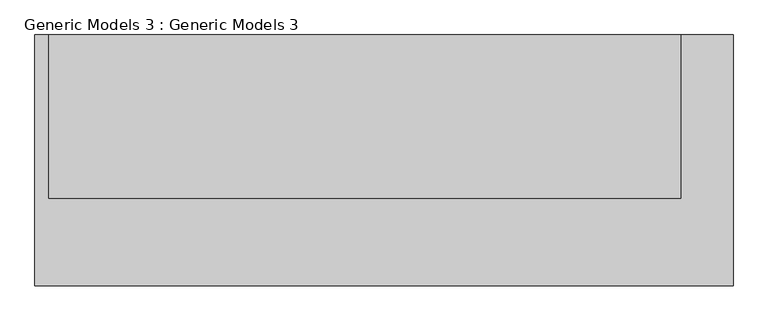
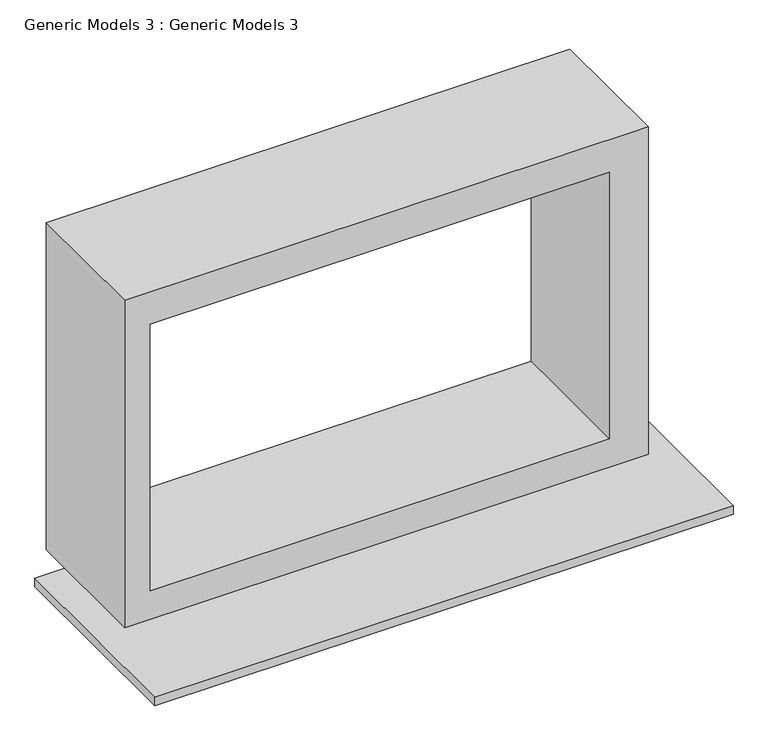
"""IFC4 building model written with IfcOpenShell, lengths in millimetres: proxy geometry, Generic Models 3 : Generic Models 3."""

from ifc_helpers import new_model, si_unit, frame, origin, place, context, project, spatial, polyline, outline, extrude, source, transform, mapped, element, save


def generic_models_3_generic_models_3_08b937b6(model_context):
    return source(origin(), model_context, "Body", "SweptSolid", [
        extrude(outline(polyline([(6400.8, -17235.5161422), (6400.8, -21845.6161422), (3352.8, -21845.6161422), (3352.8, -17235.5161422), (6400.8, -17235.5161422)]), holes=[polyline([(6096.0, -21617.0161422), (6096.0, -17578.4161422), (3616.9897637, -17578.4161422), (3616.9897637, -21617.0161422), (6096.0, -21617.0161422)])]), frame((0.0, -16095.244759, 0.0), z_axis=(0.0, 1.0, 0.0), x_axis=(0.0, 0.0, 1.0)), (0.0, 0.0, 1.0), 1191.0276278),
        extrude(outline(polyline([(-21947.2161422, -14904.2171312), (-16855.035389, -14904.2171312), (-16855.035389, -16733.0171312), (-21947.2161422, -16733.0171312), (-21947.2161422, -14904.2171312)])), frame((0.0, 0.0, 3048.0), z_axis=(0.0, 0.0, 1.0), x_axis=(1.0, 0.0, 0.0)), (0.0, 0.0, 1.0), 76.2),
    ])


if __name__ == "__main__":
    model = new_model("IFC4")
    model_context = context("Model", 3, world=origin())
    ifc_project = project(units=[si_unit("LENGTHUNIT", "METRE", prefix="MILLI")], contexts=[model_context])
    site = spatial("IfcSite", under=ifc_project)
    building = spatial("IfcBuilding", under=site)
    placement = place(None, origin())
    generic_models_3_generic_models_3_shape = generic_models_3_generic_models_3_08b937b6(model_context)
    element("IfcBuildingElementProxy", 1, Name="Generic Models 3 : Generic Models 3", ObjectType="Generic Models 3 : Generic Models 3", at=placement, inside=building, context=model_context, shape_type="MappedRepresentation", body=[
        mapped(generic_models_3_generic_models_3_shape, transform((0.0, 0.0, 0.0), x_axis=(1.0, 0.0, 0.0), y_axis=(0.0, 1.0, 0.0), z_axis=(0.0, 0.0, 1.0))),
    ])
    save(model, "model.ifc")
